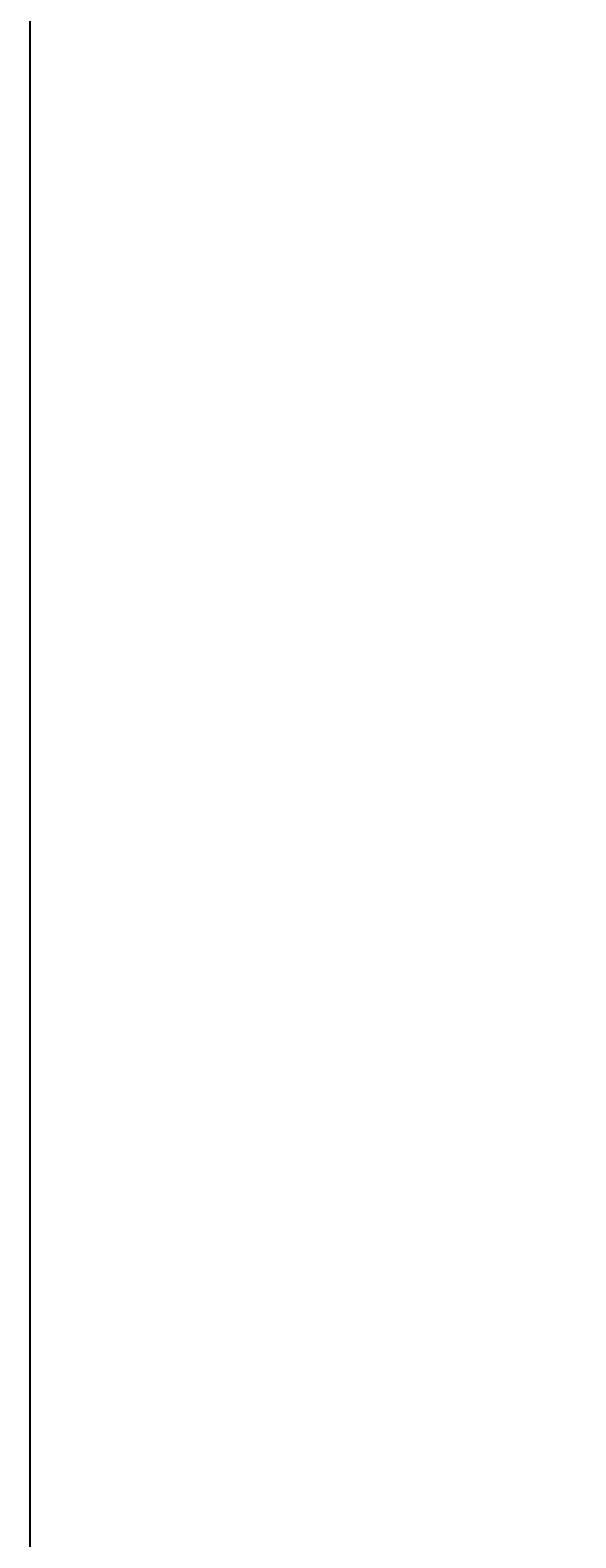
# Model space of a CAD drawing. Units: inches. Extents: x -61 to 1599, y -1316 to 257.
# Tile 129 of 204: x 372 to 388, y -122 to -77. Entities that reach past the tile are written whole.
import ezdxf

# ---------------------------------------------------------------- set-up
doc = ezdxf.new("R2010")
doc.units = ezdxf.units.IN
doc.header["$MEASUREMENT"] = 0
doc.layers.add('A-ANNO-DIMS', color=2, linetype='Continuous', lineweight=18)
doc.styles.get("Standard").update_dxf_attribs({"font": 'arial.ttf'})
doc.dimstyles.get("Standard").update_dxf_attribs({"dimtxt": 0.18, "dimasz": 0.18, "dimexe": 0.18, "dimexo": 0.0625, "dimgap": 0.09, "dimtad": 0, "dimtih": 1, "dimtoh": 1, "dimdec": 0, "dimzin": 0, "dimdsep": 46, "dimlunit": 3, "dimtxsty": 'Standard', "dimcen": 0.09, "dimadec": 0, "dimazin": 0, "dimtfac": 1, "dimtdec": 0, "dimtofl": 0, "dimtmove": 0, "dimatfit": 3, "dimfxl": 1, "dimtolj": 1, "dimtzin": 0, "dimarcsym": 0})

# ---------------------------------------------------------------- blocks, each defined once
blk = doc.blocks.new('*D703')
at = {"layer": 'A-ANNO-DIMS', "color": 0, "lineweight": -2, "transparency": 16777216}
for p, q in [((372.32, -616.882), (372.32, 257.457)), ((372.5, 257.277), (413.7, 257.277)), ((455.653, 257.277), (414.453, 257.277)), ((455.833, -616.882), (455.833, 257.457))]:
    blk.add_line(p, q, dxfattribs=at)
at = {"layer": 'A-ANNO-DIMS', "color": 0, "transparency": 16777216}
for points in [[(372.5, 257.307), (372.5, 257.247), (372.32, 257.277)], [(455.653, 257.307), (455.653, 257.247), (455.833, 257.277)]]:
    blk.add_solid(points, dxfattribs=at)
at = {"layer": 'DEFPOINTS', "color": 0, "transparency": 16777216}
for p in [(455.833, 257.277), (372.32, -616.945), (455.833, -616.945)]:
    blk.add_point(p, dxfattribs=at)
at = {"layer": 'A-ANNO-DIMS', "color": 0, "transparency": 16777216, "insert": (414.076, 257.277), "char_height": 0.18, "attachment_point": 5}
blk.add_mtext('\\A1;83.51', dxfattribs=at)

msp = doc.modelspace()

# ---------------------------------------------------------------- dimensions: what is measured, and where the dimension line sits
at = {"layer": 'A-ANNO-DIMS'}
dim = msp.add_linear_dim(base=(455.8327, 257.2771), p1=(372.3201, -616.9446), p2=(455.8327, -616.9446), dimstyle='Standard', override={"dimdec": 2, "dimlfac": 1, "dimrnd": 0, "dimzin": 0, "dimdsep": 46, "dimlunit": 2}, dxfattribs=at)
dim.commit()
dim.dimension.update_dxf_attribs({"geometry": '*D703', "text_midpoint": (414.0764, 257.2771)})

doc.saveas('drawing.dxf')
